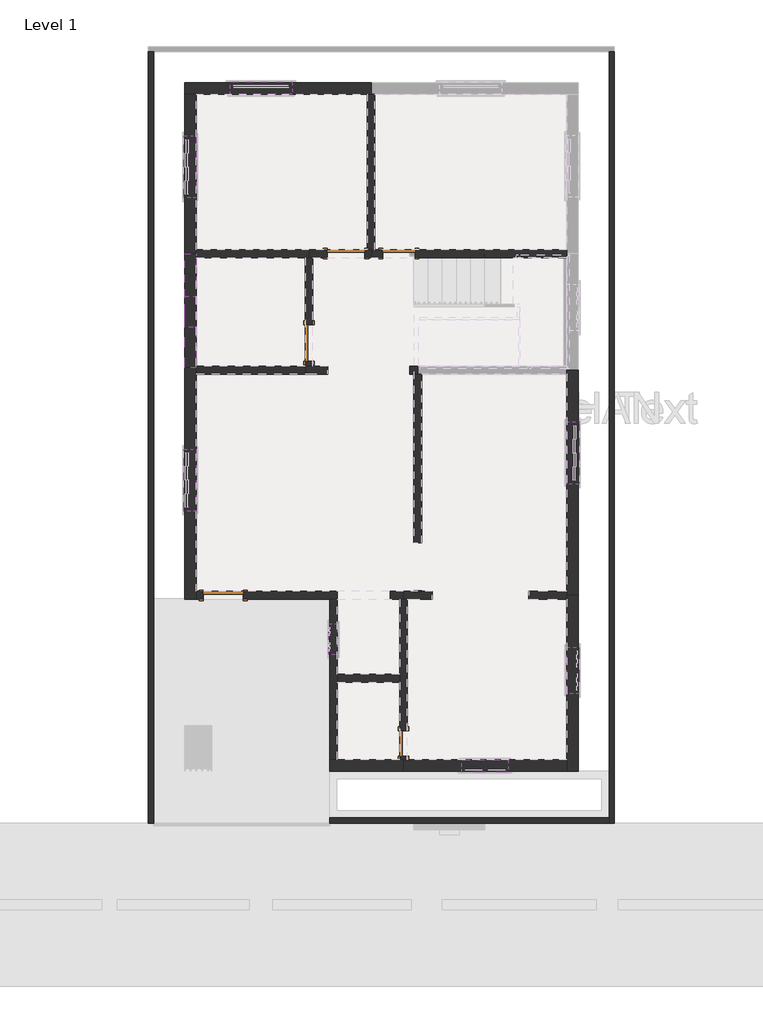
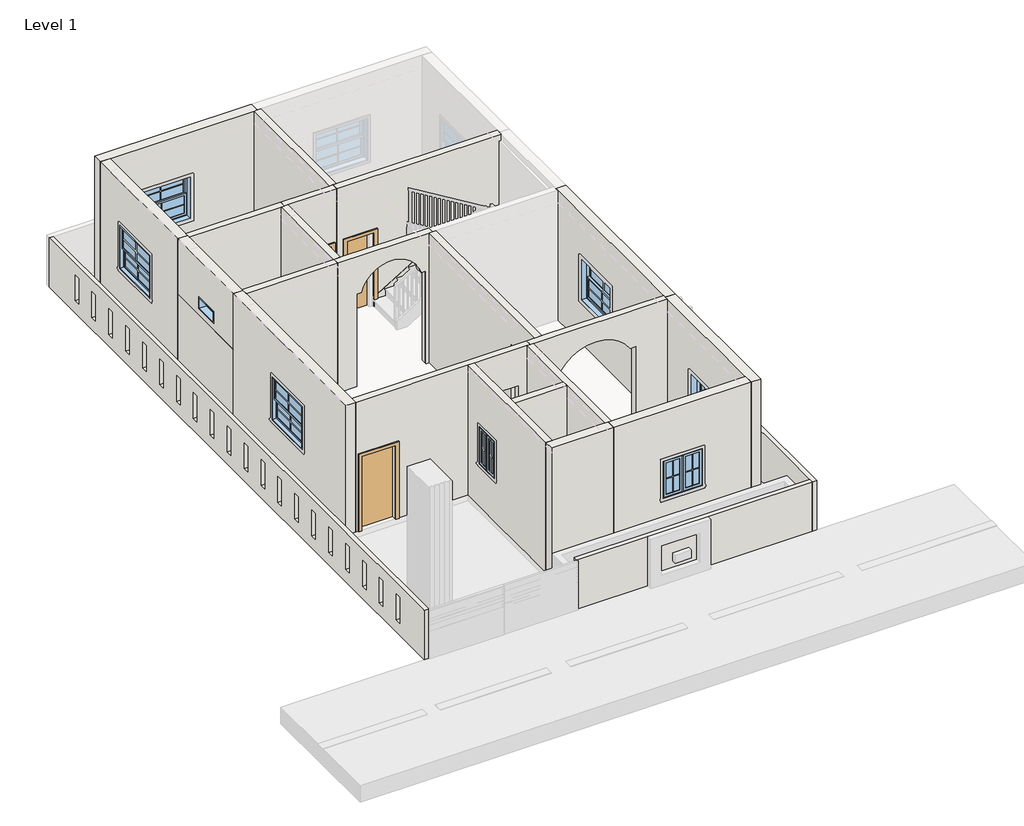
# One storey, part 1 of 3: 25 walls, 8 windows, 5 doors.
# Revit data of these elements (continued)
# Element 32 (IfcWindow, "Window-Casement-Double : 2'")
#   Mark = "9"
#   Window Inset = 0' - 0"
#   Interior Wall Closure = 0' - 2 1/4"
#   Frame Extension = 0' - 0 1/4"
#   Exterior Wall Closure = 0' - 1 1/4"
#   Interior Trim Visibility = yes
#   Exterior Trim Visibility = yes
#   Phase Created = New Construction
#   Materials on its faces: "Wood - Stained", "Glass", "Clad - White"
# Element 33 (IfcWindow, "Window-Casement-Double : 3'")
#   Mark = "7"
#   Window Inset = 0' - 0"
#   Interior Wall Closure = 0' - 2 1/4"
#   Frame Extension = 0' - 0 1/4"
#   Exterior Wall Closure = 0' - 1 1/4"
#   Interior Trim Visibility = yes
#   Exterior Trim Visibility = yes
#   Phase Created = New Construction
#   Materials on its faces: "Wood - Stained", "Glass", "Clad - White"
# Element 34 (IfcWindow, "Window-Casement-Double : 3'")
#   Mark = "8"
#   Window Inset = 0' - 0"
#   Interior Wall Closure = 0' - 2 1/4"
#   Frame Extension = 0' - 0 1/4"
#   Exterior Wall Closure = 0' - 1 1/4"
#   Interior Trim Visibility = yes
#   Exterior Trim Visibility = yes
#   Phase Created = New Construction
#   Materials on its faces: "Wood - Stained", "Glass", "Clad - White"
# Element 35 (IfcWindow, "Window-Double-Hung : 4'")
#   Mark = "3"
#   Window Inset = 0' - 0"
#   Interior Wall Closure = 0' - 1 1/2"
#   Frame Extension = 0' - 1 1/4"
#   Exterior Wall Closure = 0' - 0 1/2"
#   Interior Trim Visibility = yes
#   Indicator Visibility = yes
#   Exterior Trim Visibility = yes
#   Phase Created = New Construction
#   Materials on its faces: "Wood - Stained", "Glass", "Clad - White"
# Element 36 (IfcWindow, "Window-Double-Hung : 4'")
#   Mark = "5"
#   Window Inset = 0' - 0"
#   Interior Wall Closure = 0' - 1 1/2"
#   Frame Extension = 0' - 1 1/4"
#   Exterior Wall Closure = 0' - 0 1/2"
#   Interior Trim Visibility = yes
#   Indicator Visibility = yes
#   Exterior Trim Visibility = yes
#   Phase Created = New Construction
#   Materials on its faces: "Wood - Stained", "Glass", "Clad - White"
# Element 37 (IfcWindow, "Window-Double-Hung : 4'")
#   Mark = "6"
#   Window Inset = 0' - 0"
#   Interior Wall Closure = 0' - 1 1/2"
#   Frame Extension = 0' - 1 1/4"
#   Exterior Wall Closure = 0' - 0 1/2"
#   Interior Trim Visibility = yes
#   Indicator Visibility = yes
#   Exterior Trim Visibility = yes
#   Phase Created = New Construction
#   Materials on its faces: "Wood - Stained", "Glass", "Clad - White"
# Element 38 (IfcWindow, "Window-Double-Hung : 4'")
#   Mark = "1"
#   Window Inset = 0' - 0"
#   Interior Wall Closure = 0' - 1 1/2"
#   Frame Extension = 0' - 1 1/4"
#   Exterior Wall Closure = 0' - 0 1/2"
#   Interior Trim Visibility = yes
#   Indicator Visibility = yes
#   Exterior Trim Visibility = yes
#   Phase Created = New Construction
#   Materials on its faces: "Wood - Stained", "Glass", "Clad - White"
# Materials
#   "Door - Panel": class "Wood", colour RGB 210 159 95, transparency 0, Cost = 0
#   "Door - Frame": colour RGB 118 70 51, transparency 0, Cost = 0
#   "Glass": class "Glass", colour RGB 0 128 192, transparency 0.75, Description = "Soda Lime Glass", Cost = 0
#   "Sash": class "Wood", colour RGB 224 178 126, transparency 0, Cost = 0
#   "Wood - Stained": class "Wood", colour RGB 224 178 126, transparency 0, Cost = 0
#   "Clad - White": class "Wood", colour RGB 242 242 238, transparency 0, Cost = 0
#   "CREAM": class "Generic", colour RGB 120 120 120, transparency 0, Cost = 0
#   "Default Wall": colour RGB 128 128 128, transparency 0, Cost = 0
#   "LAVENDER WHITE": class "Generic", colour RGB 120 120 120, transparency 0, Cost = 0
#   "LIVING ROOM WALL": class "Generic", colour RGB 120 120 120, transparency 0, Cost = 0
#   "BURGUNDY COLOUR": class "Generic", colour RGB 120 120 120, transparency 0, Cost = 0
#   "DINING ROOM WALL": class "Generic", colour RGB 120 120 120, transparency 0, Cost = 0
#   "GOLD": class "Generic", colour RGB 120 120 120, transparency 0, Cost = 0
#   "BATHROOM TILES": class "Generic", colour RGB 120 120 120, transparency 0, Cost = 0
